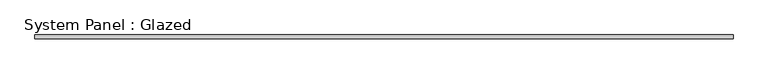
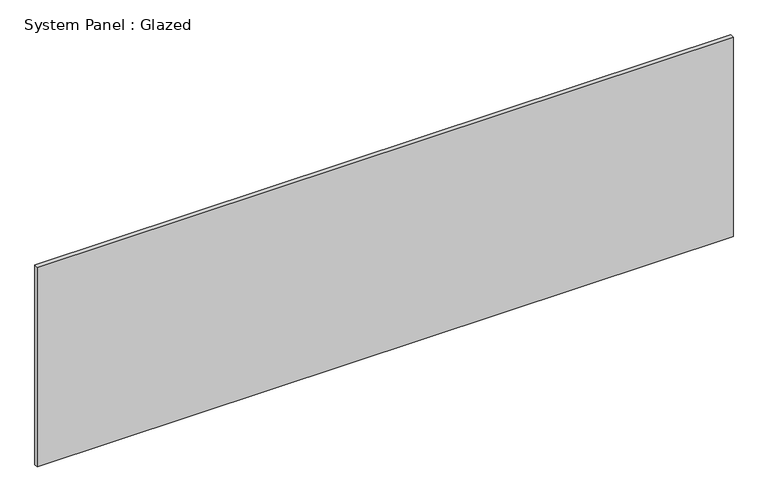
"""IFC4 building model written with IfcOpenShell, lengths in millimetres: plate geometry, System Panel : Glazed."""

from ifc_helpers import new_model, si_unit, origin, origin_with_axes, place, context, project, spatial, polyline, outline, extrude, source, transform, mapped, element, save


def system_panel_glazed_82bc3a22(model_context):
    return source(origin(), model_context, "Body", "SweptSolid", [
        extrude(outline(polyline([(2406.65, 19.05), (-2406.65, 19.05), (-2406.65, 44.45), (2406.65, 44.45), (2406.65, 19.05)])), origin_with_axes(), (0.0, 0.0, 1.0), 1460.5),
    ])


if __name__ == "__main__":
    model = new_model("IFC4")
    model_context = context("Model", 3, world=origin())
    ifc_project = project(units=[si_unit("LENGTHUNIT", "METRE", prefix="MILLI")], contexts=[model_context])
    site = spatial("IfcSite", under=ifc_project)
    building = spatial("IfcBuilding", under=site)
    placement = place(None, origin())
    system_panel_glazed_shape = system_panel_glazed_82bc3a22(model_context)
    element("IfcPlate", 1, ObjectType="System Panel : Glazed", at=placement, inside=building, context=model_context, shape_type="MappedRepresentation", body=[
        mapped(system_panel_glazed_shape, transform((0.0, 0.0, 0.0), x_axis=(1.0, 0.0, 0.0), y_axis=(0.0, 1.0, 0.0), z_axis=(0.0, 0.0, 1.0))),
    ])
    save(model, "model.ifc")

# Revit data of these elements
# Type "System Panel : Glazed"
#   Construction Type Id = "GSP4R"
#   Analytic Construction = "1/8 in Pilkington single glazing"
#   Visual Light Transmittance = 0.9
#   Solar Heat Gain Coefficient = 0.86
#   Heat Transfer Coefficient (U) = 1.18115 BTU/(h·ft²·°F)
# Element 1 (IfcPlate, "System Panel : Glazed")
#   Materials on its faces: "Glass"
# Materials
#   "Glass": class "Glass", colour RGB 0 128 192, transparency 0.75, Description = "Soda Lime Glass", Cost = 0
